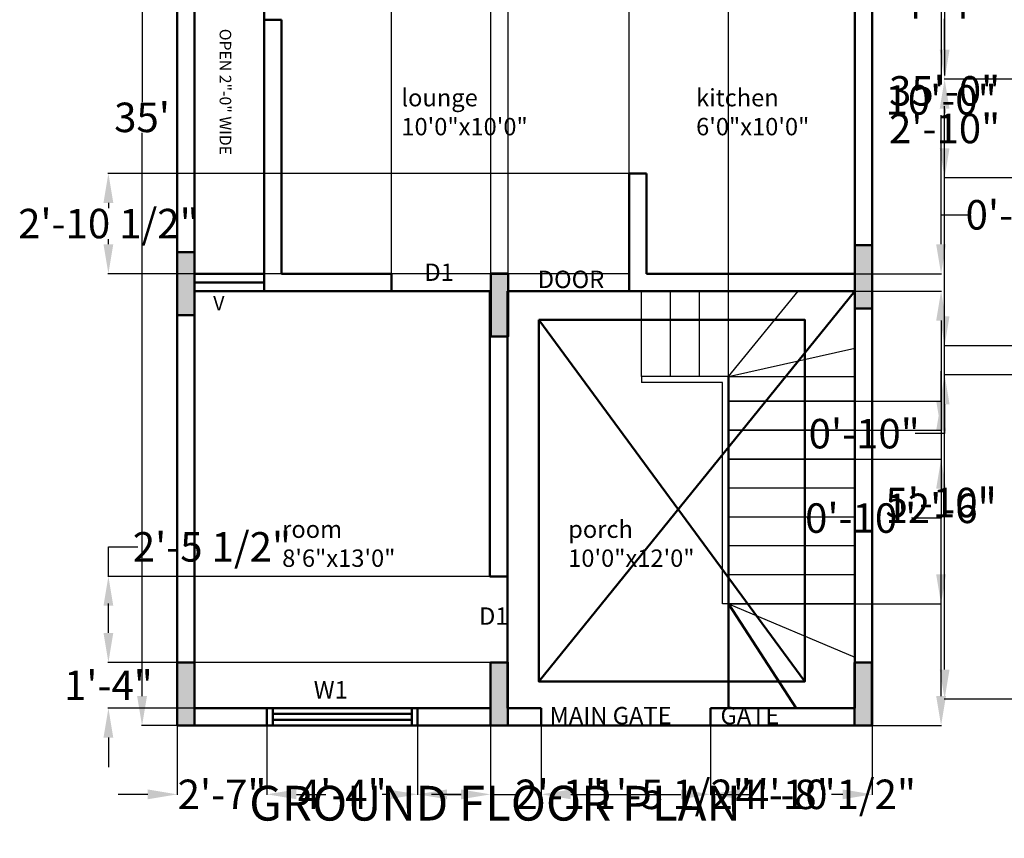
# Model space of a CAD drawing. Units: inches. Extents: x 21 to 3450, y 4 to 2137.
# Tile 1 of 14: x 2173 to 2513, y 1039 to 1321. Entities that reach past the tile are written whole.
import ezdxf

# ---------------------------------------------------------------- set-up
doc = ezdxf.new("R2010")
doc.units = ezdxf.units.IN
doc.header["$MEASUREMENT"] = 0
for name, color, linetype, lineweight in [('A-ANNO-DIMS', 2, 'Continuous', 18), ('A-ANNO-TEXT', 7, 'Continuous', 18), ('A-AREA-IDEN', 3, 'Continuous', 18), ('A-FLOR-STRS', 2, 'Continuous', 25), ('A-WALL', 7, 'Continuous', 50), ('A-WALL-PATT', 8, 'Continuous', 13)]:
    doc.layers.add(name, color=color, linetype=linetype, lineweight=lineweight)
doc.styles.get("Standard").update_dxf_attribs({"font": 'arial.ttf'})
doc.dimstyles.get("Standard").update_dxf_attribs({"dimtxt": 10.18, "dimasz": 10.18, "dimexe": 0.18, "dimexo": 0.0625, "dimgap": 0.09, "dimtad": 0, "dimtih": 1, "dimtoh": 1, "dimdec": 0, "dimzin": 0, "dimdsep": 46, "dimlunit": 3, "dimtxsty": 'Standard', "dimcen": 0.09, "dimadec": 0, "dimazin": 0, "dimtfac": 1, "dimtdec": 0, "dimtofl": 0, "dimtmove": 0, "dimatfit": 3, "dimfxl": 1, "dimtolj": 1, "dimtzin": 0, "dimarcsym": 0})

# ---------------------------------------------------------------- blocks, each defined once
blk = doc.blocks.new('*D1')
at = {"layer": 'A-ANNO-DIMS', "color": 0, "lineweight": -2, "transparency": 16777216}
for p, q in [((2227.33, 1497.5), (2215.09, 1497.5)), ((2215.27, 1487.32), (2215.27, 1292.79)), ((2215.27, 1087.68), (2215.27, 1282.21)), ((2227.33, 1077.5), (2215.09, 1077.5))]:
    blk.add_line(p, q, dxfattribs=at)
at = {"layer": 'A-ANNO-DIMS', "color": 0, "transparency": 16777216}
for points in [[(2213.57, 1487.32), (2216.97, 1487.32), (2215.27, 1497.5)], [(2213.57, 1087.68), (2216.97, 1087.68), (2215.27, 1077.5)]]:
    blk.add_solid(points, dxfattribs=at)
at = {"layer": 'Defpoints', "color": 0, "transparency": 16777216}
for p in [(2227.4, 1497.5), (2215.27, 1077.5), (2227.4, 1077.5)]:
    blk.add_point(p, dxfattribs=at)
at = {"layer": 'A-ANNO-DIMS', "color": 0, "transparency": 16777216, "insert": (2215.27, 1287.5), "char_height": 10.18, "attachment_point": 5}
blk.add_mtext("\\A1;35'", dxfattribs=at)
blk = doc.blocks.new('*D39')
at = {"layer": 'A-ANNO-DIMS', "color": 0, "lineweight": -2, "transparency": 16777216}
for p, q in [((2227.4, 1077.43), (2227.4, 1053.57)), ((2258.4, 1077.43), (2258.4, 1053.57)), ((2217.22, 1053.75), (2207.04, 1053.75)), ((2268.58, 1053.75), (2278.76, 1053.75))]:
    blk.add_line(p, q, dxfattribs=at)
at = {"layer": 'A-ANNO-DIMS', "color": 0, "transparency": 16777216}
for points in [[(2217.22, 1055.44), (2217.22, 1052.05), (2227.4, 1053.75)], [(2268.58, 1055.44), (2268.58, 1052.05), (2258.4, 1053.75)]]:
    blk.add_solid(points, dxfattribs=at)
at = {"layer": 'Defpoints', "color": 0, "transparency": 16777216}
for p in [(2227.4, 1077.5), (2258.4, 1077.5), (2258.4, 1053.75)]:
    blk.add_point(p, dxfattribs=at)
at = {"layer": 'A-ANNO-DIMS', "color": 0, "transparency": 16777216, "insert": (2242.9, 1053.75), "char_height": 10.18, "attachment_point": 5}
blk.add_mtext('\\A1;2\'-7"', dxfattribs=at)
blk = doc.blocks.new('*D40')
at = {"layer": 'A-ANNO-DIMS', "color": 0, "lineweight": -2, "transparency": 16777216}
for p, q in [((2258.4, 1077.43), (2258.4, 1053.57)), ((2310.4, 1077.43), (2310.4, 1053.57)), ((2268.58, 1053.75), (2270.57, 1053.75)), ((2300.22, 1053.75), (2298.22, 1053.75))]:
    blk.add_line(p, q, dxfattribs=at)
at = {"layer": 'A-ANNO-DIMS', "color": 0, "transparency": 16777216}
for points in [[(2268.58, 1055.44), (2268.58, 1052.05), (2258.4, 1053.75)], [(2300.22, 1055.44), (2300.22, 1052.05), (2310.4, 1053.75)]]:
    blk.add_solid(points, dxfattribs=at)
at = {"layer": 'Defpoints', "color": 0, "transparency": 16777216}
for p in [(2258.4, 1077.5), (2310.4, 1077.5), (2310.4, 1053.75)]:
    blk.add_point(p, dxfattribs=at)
at = {"layer": 'A-ANNO-DIMS', "color": 0, "transparency": 16777216, "insert": (2284.4, 1053.75), "char_height": 10.18, "attachment_point": 5}
blk.add_mtext('\\A1;4\'-4"', dxfattribs=at)
blk = doc.blocks.new('*D41')
at = {"layer": 'A-ANNO-DIMS', "color": 0, "lineweight": -2, "transparency": 16777216}
for p, q in [((2310.4, 1077.43), (2310.4, 1053.57)), ((2335.58, 1077.43), (2335.58, 1053.57)), ((2320.58, 1053.75), (2325.4, 1053.75)), ((2335.58, 1053.75), (2345.76, 1053.75))]:
    blk.add_line(p, q, dxfattribs=at)
at = {"layer": 'A-ANNO-DIMS', "color": 0, "transparency": 16777216}
for points in [[(2320.58, 1055.44), (2320.58, 1052.05), (2310.4, 1053.75)], [(2325.4, 1055.44), (2325.4, 1052.05), (2335.58, 1053.75)]]:
    blk.add_solid(points, dxfattribs=at)
at = {"layer": 'Defpoints', "color": 0, "transparency": 16777216}
for p in [(2310.4, 1077.5), (2335.58, 1077.5), (2335.58, 1053.75)]:
    blk.add_point(p, dxfattribs=at)
at = {"layer": 'A-ANNO-DIMS', "color": 0, "transparency": 16777216, "insert": (2359.46, 1053.75), "char_height": 10.18, "attachment_point": 5}
blk.add_mtext('\\A1;2\'-1"', dxfattribs=at)
blk = doc.blocks.new('*D42')
at = {"layer": 'A-ANNO-DIMS', "color": 0, "lineweight": -2, "transparency": 16777216}
for p, q in [((2353.12, 1083.43), (2353.12, 1053.57)), ((2335.58, 1077.43), (2335.58, 1053.57)), ((2325.4, 1053.75), (2315.22, 1053.75)), ((2363.3, 1053.75), (2373.48, 1053.75))]:
    blk.add_line(p, q, dxfattribs=at)
at = {"layer": 'A-ANNO-DIMS', "color": 0, "transparency": 16777216}
for points in [[(2325.4, 1055.44), (2325.4, 1052.05), (2335.58, 1053.75)], [(2363.3, 1055.44), (2363.3, 1052.05), (2353.12, 1053.75)]]:
    blk.add_solid(points, dxfattribs=at)
at = {"layer": 'Defpoints', "color": 0, "transparency": 16777216}
for p in [(2353.12, 1083.5), (2335.58, 1077.5), (2353.12, 1053.75)]:
    blk.add_point(p, dxfattribs=at)
at = {"layer": 'A-ANNO-DIMS', "color": 0, "transparency": 16777216, "insert": (2398.48, 1053.75), "char_height": 10.18, "attachment_point": 5}
blk.add_mtext('\\A1;1\'-5 1/2"', dxfattribs=at)
blk = doc.blocks.new('*D43')
at = {"layer": 'A-ANNO-DIMS', "color": 0, "lineweight": -2, "transparency": 16777216}
for p, q in [((2353.12, 1083.43), (2353.12, 1053.57)), ((2411.49, 1083.43), (2411.49, 1053.57)), ((2363.3, 1053.75), (2401.31, 1053.75)), ((2411.49, 1053.75), (2421.67, 1053.75))]:
    blk.add_line(p, q, dxfattribs=at)
at = {"layer": 'A-ANNO-DIMS', "color": 0, "transparency": 16777216}
for points in [[(2363.3, 1055.44), (2363.3, 1052.05), (2353.12, 1053.75)], [(2401.31, 1055.44), (2401.31, 1052.05), (2411.49, 1053.75)]]:
    blk.add_solid(points, dxfattribs=at)
at = {"layer": 'Defpoints', "color": 0, "transparency": 16777216}
for p in [(2353.12, 1083.5), (2411.49, 1083.5), (2411.49, 1053.75)]:
    blk.add_point(p, dxfattribs=at)
at = {"layer": 'A-ANNO-DIMS', "color": 0, "transparency": 16777216, "insert": (2451.31, 1053.75), "char_height": 10.18, "attachment_point": 5}
blk.add_mtext('\\A1;4\'-10 1/2"', dxfattribs=at)
blk = doc.blocks.new('*D44')
at = {"layer": 'A-ANNO-DIMS', "color": 0, "lineweight": -2, "transparency": 16777216}
for p, q in [((2411.49, 1083.43), (2411.49, 1053.57)), ((2467.4, 1077.43), (2467.4, 1053.57)), ((2421.67, 1053.75), (2425.62, 1053.75)), ((2457.22, 1053.75), (2453.27, 1053.75))]:
    blk.add_line(p, q, dxfattribs=at)
at = {"layer": 'A-ANNO-DIMS', "color": 0, "transparency": 16777216}
for points in [[(2421.67, 1055.44), (2421.67, 1052.05), (2411.49, 1053.75)], [(2457.22, 1055.44), (2457.22, 1052.05), (2467.4, 1053.75)]]:
    blk.add_solid(points, dxfattribs=at)
at = {"layer": 'Defpoints', "color": 0, "transparency": 16777216}
for p in [(2411.49, 1083.5), (2467.4, 1077.5), (2467.4, 1053.75)]:
    blk.add_point(p, dxfattribs=at)
at = {"layer": 'A-ANNO-DIMS', "color": 0, "transparency": 16777216, "insert": (2439.44, 1053.75), "char_height": 10.18, "attachment_point": 5}
blk.add_mtext('\\A1;4\'-8"', dxfattribs=at)
blk = doc.blocks.new('*D45')
at = {"layer": 'A-ANNO-DIMS', "color": 0, "lineweight": -2, "transparency": 16777216}
for p, q in [((2461.46, 1227.5), (2491.33, 1227.5)), ((2491.15, 1217.32), (2491.15, 1157.78)), ((2491.15, 1087.68), (2491.15, 1147.21)), ((2467.46, 1077.5), (2491.33, 1077.5))]:
    blk.add_line(p, q, dxfattribs=at)
at = {"layer": 'A-ANNO-DIMS', "color": 0, "transparency": 16777216}
for points in [[(2489.45, 1217.32), (2492.84, 1217.32), (2491.15, 1227.5)], [(2489.45, 1087.68), (2492.84, 1087.68), (2491.15, 1077.5)]]:
    blk.add_solid(points, dxfattribs=at)
at = {"layer": 'Defpoints', "color": 0, "transparency": 16777216}
for p in [(2461.4, 1227.5), (2491.15, 1227.5), (2467.4, 1077.5)]:
    blk.add_point(p, dxfattribs=at)
at = {"layer": 'A-ANNO-DIMS', "color": 0, "transparency": 16777216, "insert": (2491.15, 1152.5), "char_height": 10.18, "attachment_point": 5}
blk.add_mtext('\\A1;12\'-6"', dxfattribs=at)
blk = doc.blocks.new('*D46')
at = {"layer": 'A-ANNO-DIMS', "color": 0, "lineweight": -2, "transparency": 16777216}
for p, q in [((2491.15, 1243.68), (2491.15, 1253.86)), ((2491.15, 1253.86), (2501.33, 1253.86)), ((2461.46, 1233.5), (2491.33, 1233.5)), ((2461.46, 1227.5), (2491.33, 1227.5)), ((2491.15, 1217.32), (2491.15, 1207.14))]:
    blk.add_line(p, q, dxfattribs=at)
at = {"layer": 'A-ANNO-DIMS', "color": 0, "transparency": 16777216}
for points in [[(2489.45, 1243.68), (2492.84, 1243.68), (2491.15, 1233.5)], [(2489.45, 1217.32), (2492.84, 1217.32), (2491.15, 1227.5)]]:
    blk.add_solid(points, dxfattribs=at)
at = {"layer": 'Defpoints', "color": 0, "transparency": 16777216}
for p in [(2461.4, 1233.5), (2491.15, 1233.5), (2461.4, 1227.5)]:
    blk.add_point(p, dxfattribs=at)
at = {"layer": 'A-ANNO-DIMS', "color": 0, "transparency": 16777216, "insert": (2514.95, 1253.86), "char_height": 10.18, "attachment_point": 5}
blk.add_mtext('\\A1;0\'-6"', dxfattribs=at)
blk = doc.blocks.new('*D47')
at = {"layer": 'A-ANNO-DIMS', "color": 0, "lineweight": -2, "transparency": 16777216}
for p, q in [((2461.25, 1353.55), (2491.33, 1353.55)), ((2491.15, 1343.37), (2491.15, 1298.81)), ((2491.15, 1243.68), (2491.15, 1288.24)), ((2461.46, 1233.5), (2491.33, 1233.5))]:
    blk.add_line(p, q, dxfattribs=at)
at = {"layer": 'A-ANNO-DIMS', "color": 0, "transparency": 16777216}
for points in [[(2489.45, 1343.37), (2492.84, 1343.37), (2491.15, 1353.55)], [(2489.45, 1243.68), (2492.84, 1243.68), (2491.15, 1233.5)]]:
    blk.add_solid(points, dxfattribs=at)
at = {"layer": 'Defpoints', "color": 0, "transparency": 16777216}
for p in [(2461.19, 1353.55), (2491.15, 1353.55), (2461.4, 1233.5)]:
    blk.add_point(p, dxfattribs=at)
at = {"layer": 'A-ANNO-DIMS', "color": 0, "transparency": 16777216, "insert": (2491.15, 1293.53), "char_height": 10.18, "attachment_point": 5}
blk.add_mtext('\\A1;10\'-0"', dxfattribs=at)
blk = doc.blocks.new('*D51')
at = {"layer": 'A-ANNO-DIMS', "color": 0, "lineweight": -2, "transparency": 16777216}
for p, q in [((2383.33, 1268.16), (2203.47, 1268.16)), ((2203.65, 1257.98), (2203.65, 1256.18)), ((2203.65, 1243.68), (2203.65, 1245.48)), ((2383.33, 1233.5), (2203.47, 1233.5))]:
    blk.add_line(p, q, dxfattribs=at)
at = {"layer": 'A-ANNO-DIMS', "color": 0, "transparency": 16777216}
for points in [[(2201.95, 1257.98), (2205.34, 1257.98), (2203.65, 1268.16)], [(2201.95, 1243.68), (2205.34, 1243.68), (2203.65, 1233.5)]]:
    blk.add_solid(points, dxfattribs=at)
at = {"layer": 'Defpoints', "color": 0, "transparency": 16777216}
for p in [(2203.65, 1268.16), (2383.4, 1268.16), (2383.4, 1233.5)]:
    blk.add_point(p, dxfattribs=at)
at = {"layer": 'A-ANNO-DIMS', "color": 0, "transparency": 16777216, "insert": (2203.65, 1250.83), "char_height": 10.18, "attachment_point": 5}
blk.add_mtext('\\A1;2\'-10 1/2"', dxfattribs=at)
blk = doc.blocks.new('*D57')
at = {"layer": 'A-ANNO-DIMS', "color": 0, "lineweight": -2, "transparency": 16777216}
for p, q in [((2301.35, 1233.56), (2301.35, 1521.59)), ((2311.53, 1521.41), (2325.47, 1521.41)), ((2335.65, 1233.56), (2335.65, 1521.59)), ((2335.65, 1521.41), (2345.83, 1521.41))]:
    blk.add_line(p, q, dxfattribs=at)
at = {"layer": 'A-ANNO-DIMS', "color": 0, "transparency": 16777216}
for points in [[(2311.53, 1523.11), (2311.53, 1519.72), (2301.35, 1521.41)], [(2325.47, 1523.11), (2325.47, 1519.72), (2335.65, 1521.41)]]:
    blk.add_solid(points, dxfattribs=at)
at = {"layer": 'Defpoints', "color": 0, "transparency": 16777216}
for p in [(2335.65, 1521.41), (2301.35, 1233.5), (2335.65, 1233.5)]:
    blk.add_point(p, dxfattribs=at)
at = {"layer": 'A-ANNO-DIMS', "color": 0, "transparency": 16777216, "insert": (2375.36, 1521.41), "char_height": 10.18, "attachment_point": 5}
blk.add_mtext('\\A1;2\'-10 1/2"', dxfattribs=at)
blk = doc.blocks.new('*D58')
at = {"layer": 'A-ANNO-DIMS', "color": 0, "lineweight": -2, "transparency": 16777216}
for p, q in [((2341.65, 1233.56), (2341.65, 1521.59)), ((2351.83, 1521.41), (2373.22, 1521.41)), ((2383.4, 1233.56), (2383.4, 1521.59)), ((2383.4, 1521.41), (2393.58, 1521.41))]:
    blk.add_line(p, q, dxfattribs=at)
at = {"layer": 'A-ANNO-DIMS', "color": 0, "transparency": 16777216}
for points in [[(2351.83, 1523.11), (2351.83, 1519.72), (2341.65, 1521.41)], [(2373.22, 1523.11), (2373.22, 1519.72), (2383.4, 1521.41)]]:
    blk.add_solid(points, dxfattribs=at)
at = {"layer": 'Defpoints', "color": 0, "transparency": 16777216}
for p in [(2383.4, 1521.41), (2341.65, 1233.5), (2383.4, 1233.5)]:
    blk.add_point(p, dxfattribs=at)
at = {"layer": 'A-ANNO-DIMS', "color": 0, "transparency": 16777216, "insert": (2419.05, 1521.41), "char_height": 10.18, "attachment_point": 5}
blk.add_mtext('\\A1;3\'-5 1/2"', dxfattribs=at)
blk = doc.blocks.new('*D59')
at = {"layer": 'A-ANNO-DIMS', "color": 0, "lineweight": -2, "transparency": 16777216}
for p, q in [((2203.65, 1129.02), (2203.65, 1139.2)), ((2203.65, 1139.2), (2213.83, 1139.2)), ((2335.33, 1129.02), (2203.47, 1129.02)), ((2203.65, 1109.46), (2203.65, 1118.84)), ((2335.51, 1099.28), (2203.47, 1099.28))]:
    blk.add_line(p, q, dxfattribs=at)
at = {"layer": 'A-ANNO-DIMS', "color": 0, "transparency": 16777216}
for points in [[(2201.95, 1118.84), (2205.34, 1118.84), (2203.65, 1129.02)], [(2201.95, 1109.46), (2205.34, 1109.46), (2203.65, 1099.28)]]:
    blk.add_solid(points, dxfattribs=at)
at = {"layer": 'Defpoints', "color": 0, "transparency": 16777216}
for p in [(2203.65, 1129.02), (2335.4, 1129.02), (2335.58, 1099.28)]:
    blk.add_point(p, dxfattribs=at)
at = {"layer": 'A-ANNO-DIMS', "color": 0, "transparency": 16777216, "insert": (2239.39, 1139.2), "char_height": 10.18, "attachment_point": 5}
blk.add_mtext('\\A1;2\'-5 1/2"', dxfattribs=at)
blk = doc.blocks.new('*D60')
at = {"layer": 'A-ANNO-DIMS', "color": 0, "lineweight": -2, "transparency": 16777216}
for p, q in [((2203.65, 1109.46), (2203.65, 1119.64)), ((2335.51, 1099.28), (2203.47, 1099.28)), ((2335.33, 1083.5), (2203.47, 1083.5)), ((2203.65, 1073.32), (2203.65, 1063.14))]:
    blk.add_line(p, q, dxfattribs=at)
at = {"layer": 'A-ANNO-DIMS', "color": 0, "transparency": 16777216}
for points in [[(2201.95, 1109.46), (2205.34, 1109.46), (2203.65, 1099.28)], [(2201.95, 1073.32), (2205.34, 1073.32), (2203.65, 1083.5)]]:
    blk.add_solid(points, dxfattribs=at)
at = {"layer": 'Defpoints', "color": 0, "transparency": 16777216}
for p in [(2203.65, 1099.28), (2335.58, 1099.28), (2335.4, 1083.5)]:
    blk.add_point(p, dxfattribs=at)
at = {"layer": 'A-ANNO-DIMS', "color": 0, "transparency": 16777216, "insert": (2203.65, 1091.39), "char_height": 10.18, "attachment_point": 5}
blk.add_mtext('\\A1;1\'-4"', dxfattribs=at)
blk = doc.blocks.new('*D63')
at = {"layer": 'A-ANNO-DIMS', "color": 0, "lineweight": -2, "transparency": 16777216}
for p, q in [((2417.71, 1189.56), (2417.71, 1521.59)), ((2427.89, 1521.41), (2451.22, 1521.41)), ((2461.4, 1189.56), (2461.4, 1521.59)), ((2461.4, 1521.41), (2471.58, 1521.41))]:
    blk.add_line(p, q, dxfattribs=at)
at = {"layer": 'A-ANNO-DIMS', "color": 0, "transparency": 16777216}
for points in [[(2427.89, 1523.11), (2427.89, 1519.72), (2417.71, 1521.41)], [(2451.22, 1523.11), (2451.22, 1519.72), (2461.4, 1521.41)]]:
    blk.add_solid(points, dxfattribs=at)
at = {"layer": 'Defpoints', "color": 0, "transparency": 16777216}
for p in [(2461.4, 1521.41), (2417.71, 1189.5), (2461.4, 1189.5)]:
    blk.add_point(p, dxfattribs=at)
at = {"layer": 'A-ANNO-DIMS', "color": 0, "transparency": 16777216, "insert": (2497.05, 1521.41), "char_height": 10.18, "attachment_point": 5}
blk.add_mtext('\\A1;3\'-7 1/2"', dxfattribs=at)
blk = doc.blocks.new('*D64')
at = {"layer": 'A-ANNO-DIMS', "color": 0, "lineweight": -2, "transparency": 16777216}
for p, q in [((2491.15, 1189.68), (2491.15, 1199.86)), ((2417.77, 1179.5), (2491.33, 1179.5)), ((2417.77, 1169.5), (2491.33, 1169.5)), ((2491.15, 1159.32), (2491.15, 1149.14)), ((2491.15, 1149.14), (2480.97, 1149.14))]:
    blk.add_line(p, q, dxfattribs=at)
at = {"layer": 'A-ANNO-DIMS', "color": 0, "transparency": 16777216}
for points in [[(2489.45, 1189.68), (2492.84, 1189.68), (2491.15, 1179.5)], [(2489.45, 1159.32), (2492.84, 1159.32), (2491.15, 1169.5)]]:
    blk.add_solid(points, dxfattribs=at)
at = {"layer": 'Defpoints', "color": 0, "transparency": 16777216}
for p in [(2417.71, 1179.5), (2417.71, 1169.5), (2491.15, 1169.5)]:
    blk.add_point(p, dxfattribs=at)
at = {"layer": 'A-ANNO-DIMS', "color": 0, "transparency": 16777216, "insert": (2463.39, 1149.14), "char_height": 10.18, "attachment_point": 5}
blk.add_mtext('\\A1;0\'-10"', dxfattribs=at)
blk = doc.blocks.new('*D65')
at = {"layer": 'A-ANNO-DIMS', "color": 0, "lineweight": -2, "transparency": 16777216}
for p, q in [((2417.77, 1189.5), (2491.33, 1189.5)), ((2491.15, 1179.32), (2491.15, 1159.78)), ((2491.15, 1129.68), (2491.15, 1149.21)), ((2417.77, 1119.5), (2491.33, 1119.5))]:
    blk.add_line(p, q, dxfattribs=at)
at = {"layer": 'A-ANNO-DIMS', "color": 0, "transparency": 16777216}
for points in [[(2489.45, 1179.32), (2492.84, 1179.32), (2491.15, 1189.5)], [(2489.45, 1129.68), (2492.84, 1129.68), (2491.15, 1119.5)]]:
    blk.add_solid(points, dxfattribs=at)
at = {"layer": 'Defpoints', "color": 0, "transparency": 16777216}
for p in [(2417.71, 1189.5), (2417.71, 1119.5), (2491.15, 1119.5)]:
    blk.add_point(p, dxfattribs=at)
at = {"layer": 'A-ANNO-DIMS', "color": 0, "transparency": 16777216, "insert": (2491.15, 1154.5), "char_height": 10.18, "attachment_point": 5}
blk.add_mtext('\\A1;5\'-10"', dxfattribs=at)
blk = doc.blocks.new('*D67')
at = {"layer": 'A-ANNO-DIMS', "color": 0, "lineweight": -2, "transparency": 16777216}
for p, q in [((2515.64, 1506.65), (2492.19, 1506.65)), ((2492.37, 1496.47), (2492.37, 1301.94)), ((2492.37, 1096.83), (2492.37, 1291.36)), ((2515.56, 1086.65), (2492.19, 1086.65))]:
    blk.add_line(p, q, dxfattribs=at)
at = {"layer": 'A-ANNO-DIMS', "color": 0, "transparency": 16777216}
for points in [[(2490.67, 1496.47), (2494.06, 1496.47), (2492.37, 1506.65)], [(2490.67, 1096.83), (2494.06, 1096.83), (2492.37, 1086.65)]]:
    blk.add_solid(points, dxfattribs=at)
at = {"layer": 'Defpoints', "color": 0, "transparency": 16777216}
for p in [(2492.37, 1506.65), (2515.71, 1506.65), (2515.62, 1086.65)]:
    blk.add_point(p, dxfattribs=at)
at = {"layer": 'A-ANNO-DIMS', "color": 0, "transparency": 16777216, "insert": (2492.37, 1296.65), "char_height": 10.18, "attachment_point": 5}
blk.add_mtext('\\A1;35\'-0"', dxfattribs=at)
blk = doc.blocks.new('*D89')
at = {"layer": 'A-ANNO-DIMS', "color": 0, "lineweight": -2, "transparency": 16777216}
for p, q in [((2545.64, 1352.65), (2492.19, 1352.65)), ((2492.37, 1342.47), (2492.37, 1331.83)), ((2492.37, 1310.83), (2492.37, 1321.47)), ((2545.64, 1300.65), (2492.19, 1300.65))]:
    blk.add_line(p, q, dxfattribs=at)
at = {"layer": 'A-ANNO-DIMS', "color": 0, "transparency": 16777216}
for points in [[(2490.67, 1342.47), (2494.06, 1342.47), (2492.37, 1352.65)], [(2490.67, 1310.83), (2494.06, 1310.83), (2492.37, 1300.65)]]:
    blk.add_solid(points, dxfattribs=at)
at = {"layer": 'Defpoints', "color": 0, "transparency": 16777216}
for p in [(2492.37, 1352.65), (2545.71, 1352.65), (2545.71, 1300.65)]:
    blk.add_point(p, dxfattribs=at)
at = {"layer": 'A-ANNO-DIMS', "color": 0, "transparency": 16777216, "insert": (2492.37, 1326.65), "char_height": 10.18, "attachment_point": 5}
blk.add_mtext('\\A1;4\'-4"', dxfattribs=at)
blk = doc.blocks.new('*D90')
at = {"layer": 'A-ANNO-DIMS', "color": 0, "lineweight": -2, "transparency": 16777216}
for p, q in [((2545.64, 1300.65), (2492.19, 1300.65)), ((2492.37, 1290.47), (2492.37, 1288.94)), ((2492.37, 1276.83), (2492.37, 1278.36)), ((2545.64, 1266.65), (2492.19, 1266.65))]:
    blk.add_line(p, q, dxfattribs=at)
at = {"layer": 'A-ANNO-DIMS', "color": 0, "transparency": 16777216}
for points in [[(2490.67, 1290.47), (2494.06, 1290.47), (2492.37, 1300.65)], [(2490.67, 1276.83), (2494.06, 1276.83), (2492.37, 1266.65)]]:
    blk.add_solid(points, dxfattribs=at)
at = {"layer": 'Defpoints', "color": 0, "transparency": 16777216}
for p in [(2492.37, 1300.65), (2545.71, 1300.65), (2545.71, 1266.65)]:
    blk.add_point(p, dxfattribs=at)
at = {"layer": 'A-ANNO-DIMS', "color": 0, "transparency": 16777216, "insert": (2492.37, 1283.65), "char_height": 10.18, "attachment_point": 5}
blk.add_mtext('\\A1;2\'-10"', dxfattribs=at)
blk = doc.blocks.new('*D94')
at = {"layer": 'A-ANNO-DIMS', "color": 0, "lineweight": -2, "transparency": 16777216}
for p, q in [((2492.37, 1218.83), (2492.37, 1229.01)), ((2707.42, 1208.65), (2492.19, 1208.65)), ((2707.42, 1198.65), (2492.19, 1198.65)), ((2492.37, 1188.47), (2492.37, 1178.29)), ((2492.37, 1178.29), (2482.19, 1178.29))]:
    blk.add_line(p, q, dxfattribs=at)
at = {"layer": 'A-ANNO-DIMS', "color": 0, "transparency": 16777216}
for points in [[(2490.67, 1218.83), (2494.06, 1218.83), (2492.37, 1208.65)], [(2490.67, 1188.47), (2494.06, 1188.47), (2492.37, 1198.65)]]:
    blk.add_solid(points, dxfattribs=at)
at = {"layer": 'Defpoints', "color": 0, "transparency": 16777216}
for p in [(2707.48, 1208.65), (2492.37, 1198.65), (2707.48, 1198.65)]:
    blk.add_point(p, dxfattribs=at)
at = {"layer": 'A-ANNO-DIMS', "color": 0, "transparency": 16777216, "insert": (2464.61, 1178.29), "char_height": 10.18, "attachment_point": 5}
blk.add_mtext('\\A1;0\'-10"', dxfattribs=at)

msp = doc.modelspace()

# ---------------------------------------------------------------- hatches: boundary and pattern name
at = {"layer": 'A-WALL-PATT'}
h = msp.add_hatch(color=256, dxfattribs=at)
h.dxf.hatch_style = 1
h.paths.add_polyline_path([(2233.4, 1497.5), (2227.4, 1497.5), (2227.4, 1475.71), (2233.4, 1475.71)])
h.paths.add_polyline_path([(2322.77, 1497.5), (2300.98, 1497.5), (2300.98, 1491.66), (2322.77, 1491.66)])
h.paths.add_polyline_path([(2467.26, 1497.5), (2461.26, 1497.5), (2461.26, 1491.5), (2461.4, 1491.5), (2461.4, 1475.76), (2467.26, 1475.76)])
h.paths.add_polyline_path([(2233.4, 1369.46), (2227.4, 1369.46), (2227.4, 1347.68), (2233.4, 1347.68)])
h.paths.add_polyline_path([(2314.37, 1375.28), (2308.4, 1375.28), (2308.4, 1359.5), (2308.37, 1353.5), (2314.37, 1353.5)])
h.paths.add_polyline_path([(2467.19, 1375.34), (2461.4, 1375.34), (2461.4, 1359.5), (2461.19, 1353.55), (2467.19, 1353.55)])
h.paths.add_polyline_path([(2467.34, 1243.32), (2461.4, 1243.32), (2461.4, 1233.5), (2461.37, 1227.5), (2461.4, 1227.5), (2461.4, 1221.53), (2467.34, 1221.53)])
h.paths.add_polyline_path([(2341.4, 1227.5), (2341.65, 1227.5), (2341.65, 1233.5), (2335.65, 1233.5), (2335.65, 1211.8), (2341.4, 1211.8)])
h.paths.add_polyline_path([(2233.4, 1241.01), (2227.4, 1241.01), (2227.4, 1219.23), (2233.4, 1219.23)])
h.paths.add_polyline_path([(2341.4, 1099.28), (2335.58, 1099.28), (2335.58, 1077.5), (2341.58, 1077.5), (2341.58, 1083.5), (2341.4, 1083.5)])
h.paths.add_polyline_path([(2467.29, 1099.28), (2461.4, 1099.28), (2461.4, 1083.5), (2461.29, 1077.5), (2467.29, 1077.5)])
h = msp.add_hatch(color=256, dxfattribs=at)
h.dxf.hatch_style = 1
h.paths.add_polyline_path([(2233.4, 1099.28), (2227.4, 1099.28), (2227.4, 1077.5), (2233.4, 1077.5)])

# ---------------------------------------------------------------- linework, layer by layer
at = {"layer": 'A-FLOR-STRS'}
for p, q in [((2387.71, 1198), (2387.71, 1227.5)), ((2397.71, 1198), (2397.71, 1227.5)), ((2407.71, 1198), (2407.71, 1227.5)), ((2417.71, 1198), (2417.71, 1227.5)), ((2417.71, 1198), (2441.78, 1227.5)), ((2417.71, 1198), (2461.4, 1207.86)), ((2417.71, 1198), (2387.71, 1198)), ((2387.71, 1198), (2387.71, 1196)), ((2417.71, 1198), (2461.4, 1198)), ((2415.71, 1196), (2387.71, 1196)), ((2415.71, 1119.5), (2415.71, 1196)), ((2461.4, 1189.5), (2417.71, 1189.5)), ((2461.4, 1179.5), (2417.71, 1179.5)), ((2461.4, 1169.5), (2417.71, 1169.5)), ((2461.4, 1159.5), (2417.71, 1159.5)), ((2461.4, 1149.5), (2417.71, 1149.5)), ((2461.4, 1139.5), (2417.71, 1139.5)), ((2461.4, 1129.5), (2417.71, 1129.5)), ((2417.71, 1119.5), (2415.71, 1119.5)), ((2461.4, 1119.5), (2417.71, 1119.5)), ((2417.71, 1119.5), (2461.4, 1101.07))]:
    msp.add_line(p, q, dxfattribs=at)
at = {"layer": 'A-WALL'}
for p, q in [((2227.4, 1077.5), (2227.4, 1497.5)), ((2467.4, 1497.5), (2467.4, 1077.5)), ((2233.4, 1233.5), (2233.4, 1353.5)), ((2257.4, 1353.5), (2257.4, 1233.5)), ((2461.4, 1353.5), (2461.4, 1233.5)), ((2257.4, 1321.23), (2263.4, 1321.23)), ((2263.4, 1321.23), (2263.4, 1233.5)), ((2383.4, 1268.16), (2389.4, 1268.16)), ((2383.4, 1268.16), (2383.4, 1233.5)), ((2389.4, 1268.16), (2389.4, 1233.5)), ((2233.4, 1233.5), (2257.4, 1233.5)), ((2233.4, 1233.5), (2233.4, 1227.5)), ((2257.4, 1233.5), (2257.4, 1227.5)), ((2263.4, 1233.5), (2301.35, 1233.5)), ((2301.35, 1233.5), (2301.35, 1227.5)), ((2335.65, 1233.5), (2341.65, 1233.5)), ((2383.4, 1233.5), (2383.4, 1227.5)), ((2389.4, 1233.5), (2461.4, 1233.5)), ((2233.4, 1230.5), (2257.4, 1230.5)), ((2233.4, 1083.5), (2233.4, 1227.5)), ((2233.4, 1227.5), (2335.4, 1227.5)), ((2335.4, 1129.02), (2335.4, 1227.5)), ((2341.4, 1083.5), (2341.4, 1227.5)), ((2341.4, 1227.5), (2461.4, 1227.5)), ((2352.29, 1092.71), (2461.4, 1227.5)), ((2461.4, 1227.5), (2461.4, 1083.5)), ((2352.29, 1217.65), (2444.07, 1092.71)), ((2417.71, 1083.5), (2417.71, 1198)), ((2335.4, 1129.02), (2341.4, 1129.02)), ((2417.71, 1119.5), (2441.17, 1083.5)), ((2335.4, 1083.5), (2233.4, 1083.5)), ((2258.4, 1083.5), (2258.4, 1077.5)), ((2260.4, 1083.5), (2260.4, 1077.5)), ((2260.4, 1081.5), (2308.4, 1081.5)), ((2308.4, 1083.5), (2308.4, 1077.5)), ((2310.4, 1083.5), (2310.4, 1077.5)), ((2353.12, 1083.5), (2341.4, 1083.5)), ((2353.12, 1083.5), (2353.12, 1077.5)), ((2417.71, 1083.5), (2411.49, 1083.5)), ((2411.49, 1083.5), (2411.49, 1077.5)), ((2461.4, 1083.5), (2417.71, 1083.5)), ((2260.4, 1079.5), (2308.4, 1079.5)), ((2467.4, 1077.5), (2227.4, 1077.5))]:
    msp.add_line(p, q, dxfattribs=at)
for points in [[(2227.4, 1241.01), (2233.4, 1241.01), (2233.4, 1219.23), (2227.4, 1219.23)], [(2461.34, 1243.32), (2467.34, 1243.32), (2467.34, 1221.53), (2461.34, 1221.53)], [(2335.65, 1233.59), (2341.65, 1233.59), (2341.65, 1211.8), (2335.65, 1211.8)], [(2352.29, 1217.65), (2444.07, 1217.65), (2444.07, 1092.71), (2352.29, 1092.71)], [(2227.4, 1099.28), (2233.4, 1099.28), (2233.4, 1077.5), (2227.4, 1077.5)], [(2335.58, 1099.28), (2341.58, 1099.28), (2341.58, 1077.5), (2335.58, 1077.5)], [(2461.29, 1099.28), (2467.29, 1099.28), (2467.29, 1077.5), (2461.29, 1077.5)]]:
    msp.add_lwpolyline(points, close=True, dxfattribs=at)

# ---------------------------------------------------------------- texts
at = {"layer": 'A-ANNO-TEXT', "insert": (2246.05, 1318.09), "char_height": 4, "attachment_point": 1, "rotation": 270}
msp.add_mtext_dynamic_manual_height_columns('OPEN 2"-0" WIDE', width=50.8458, gutter_width=1, heights=[0], dxfattribs=at)
at = {"layer": 'A-ANNO-TEXT', "attachment_point": 1}
for s, width, insert, char_height in [('D1', 23.0829, (2312.75, 1237.04), 6), ('DOOR', 23.0829, (2351.89, 1234.56), 6), ('V', 12.1398, (2239.82, 1225.84), 5), ('D1', 23.0829, (2331.62, 1118.3), 6), ('W1', 23.0829, (2274.55, 1092.83), 6), ('MAIN GATE', 46.3152, (2355.99, 1083.92), 6), (' GATE', 46.3152, (2413.14, 1083.92), 6), ('GROUND FLOOR PLAN', 189.6067, (2252.27, 1056.69), 12)]:
    msp.add_mtext_dynamic_manual_height_columns(s, width=width, gutter_width=1, heights=[0], dxfattribs=dict(at, insert=insert, char_height=char_height))
at = {"layer": 'A-AREA-IDEN', "char_height": 6, "attachment_point": 1}
for s, insert in [('lounge \\P10\'0"x10\'0"', (2304.79, 1297.31)), ('kitchen 6\'0"x10\'0"', (2406.56, 1297.31)), ('room\\P8\'6"x13\'0"', (2263.65, 1148.3)), ('porch \\P10\'0"x12\'0" ', (2362.39, 1148.3))]:
    msp.add_mtext_dynamic_manual_height_columns(s, width=31.1036, gutter_width=1, heights=[0], dxfattribs=dict(at, insert=insert))

# ---------------------------------------------------------------- dimensions: what is measured, and where the dimension line sits
at = {"layer": 'A-ANNO-DIMS'}
for base, p1, p2, picture, middle in [((2335.65, 1521.41), (2301.35, 1233.5), (2335.65, 1233.5), '*D57', (2375.36, 1521.41)), ((2383.3966, 1521.4135), (2341.6544, 1233.4971), (2383.3966, 1233.4971), '*D58', (2419.0541, 1521.4135)), ((2461.4, 1521.41), (2417.71, 1189.5), (2461.4, 1189.5), '*D63', (2497.05, 1521.41)), ((2353.12, 1053.75), (2335.58, 1077.5), (2353.12, 1083.5), '*D42', (2398.48, 1053.75)), ((2411.49, 1053.75), (2353.12, 1083.5), (2411.49, 1083.5), '*D43', (2451.31, 1053.75)), ((2467.4, 1053.75), (2411.49, 1083.5), (2467.4, 1077.5), '*D44', (2439.44, 1053.75)), ((2258.4, 1053.75), (2227.4, 1077.5), (2258.4, 1077.5), '*D39', (2242.9, 1053.75)), ((2310.4, 1053.75), (2258.4, 1077.5), (2310.4, 1077.5), '*D40', (2284.4, 1053.75)), ((2335.58, 1053.75), (2310.4, 1077.5), (2335.58, 1077.5), '*D41', (2359.46, 1053.75))]:
    dim = msp.add_linear_dim(base=base, p1=p1, p2=p2, dimstyle='Standard', override={"dimdec": 1, "dimlfac": 1, "dimrnd": 0, "dimzin": 1, "dimdsep": 46, "dimlunit": 4, "dimfrac": 2}, dxfattribs=at)
    dim.commit()
    dim.dimension.update_dxf_attribs({"geometry": picture, "text_midpoint": middle})
for base, p1, p2, override, picture, middle in [((2492.37, 1506.65), (2515.62, 1086.65), (2515.71, 1506.65), {"dimdec": 1, "dimlfac": 1, "dimrnd": 0, "dimzin": 1, "dimdsep": 46, "dimlunit": 4, "dimfrac": 2}, '*D67', (2492.37, 1296.65)), ((2215.27, 1077.5), (2227.4, 1497.5), (2227.4, 1077.5), {"dimclrd": 0, "dimclre": 0, "dimclrt": 0}, '*D1', (2215.27, 1287.5)), ((2491.1466, 1353.5544), (2461.3966, 1233.4971), (2461.1914, 1353.5544), {"dimdec": 1, "dimlfac": 1, "dimrnd": 0, "dimzin": 1, "dimdsep": 46, "dimlunit": 4, "dimfrac": 2}, '*D47', (2491.1466, 1293.5257)), ((2492.37, 1352.65), (2545.71, 1300.65), (2545.71, 1352.65), {"dimdec": 1, "dimlfac": 1, "dimrnd": 0, "dimzin": 1, "dimdsep": 46, "dimlunit": 4, "dimfrac": 2}, '*D89', (2492.37, 1326.65)), ((2492.37, 1300.65), (2545.71, 1266.65), (2545.71, 1300.65), {"dimdec": 1, "dimlfac": 1, "dimrnd": 0, "dimzin": 1, "dimdsep": 46, "dimlunit": 4, "dimfrac": 2}, '*D90', (2492.37, 1283.65)), ((2203.65, 1268.16), (2383.4, 1233.5), (2383.4, 1268.16), {"dimdec": 1, "dimlfac": 1, "dimrnd": 0, "dimzin": 1, "dimdsep": 46, "dimlunit": 4, "dimfrac": 2}, '*D51', (2203.65, 1250.83)), ((2491.15, 1233.5), (2461.4, 1227.5), (2461.4, 1233.5), {"dimdec": 1, "dimlfac": 1, "dimrnd": 0, "dimzin": 1, "dimdsep": 46, "dimlunit": 4, "dimfrac": 2}, '*D46', (2514.95, 1253.86)), ((2492.37, 1198.65), (2707.48, 1208.65), (2707.48, 1198.65), {"dimdec": 1, "dimlfac": 1, "dimrnd": 0, "dimzin": 1, "dimdsep": 46, "dimlunit": 4, "dimfrac": 2}, '*D94', (2464.61, 1178.29)), ((2491.15, 1227.5), (2467.4, 1077.5), (2461.4, 1227.5), {"dimdec": 1, "dimlfac": 1, "dimrnd": 0, "dimzin": 1, "dimdsep": 46, "dimlunit": 4, "dimfrac": 2}, '*D45', (2491.15, 1152.5)), ((2491.15, 1169.5), (2417.71, 1179.5), (2417.71, 1169.5), {"dimdec": 1, "dimlfac": 1, "dimrnd": 0, "dimzin": 1, "dimdsep": 46, "dimlunit": 4, "dimfrac": 2}, '*D64', (2463.39, 1149.14)), ((2491.15, 1119.5), (2417.71, 1189.5), (2417.71, 1119.5), {"dimdec": 1, "dimlfac": 1, "dimrnd": 0, "dimzin": 1, "dimdsep": 46, "dimlunit": 4, "dimfrac": 2}, '*D65', (2491.15, 1154.5)), ((2203.65, 1129.02), (2335.58, 1099.28), (2335.4, 1129.02), {"dimdec": 1, "dimlfac": 1, "dimrnd": 0, "dimzin": 1, "dimdsep": 46, "dimlunit": 4, "dimfrac": 2}, '*D59', (2239.39, 1139.2)), ((2203.65, 1099.28), (2335.4, 1083.5), (2335.58, 1099.28), {"dimdec": 1, "dimlfac": 1, "dimrnd": 0, "dimzin": 1, "dimdsep": 46, "dimlunit": 4, "dimfrac": 2}, '*D60', (2203.65, 1091.39))]:
    dim = msp.add_linear_dim(base=base, p1=p1, p2=p2, angle=90, dimstyle='Standard', override=override, dxfattribs=at)
    dim.commit()
    dim.dimension.update_dxf_attribs({"geometry": picture, "text_midpoint": middle})

doc.saveas('drawing.dxf')
